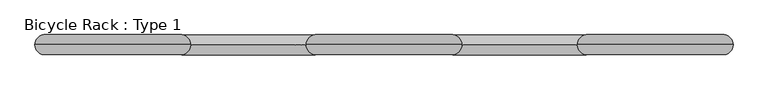
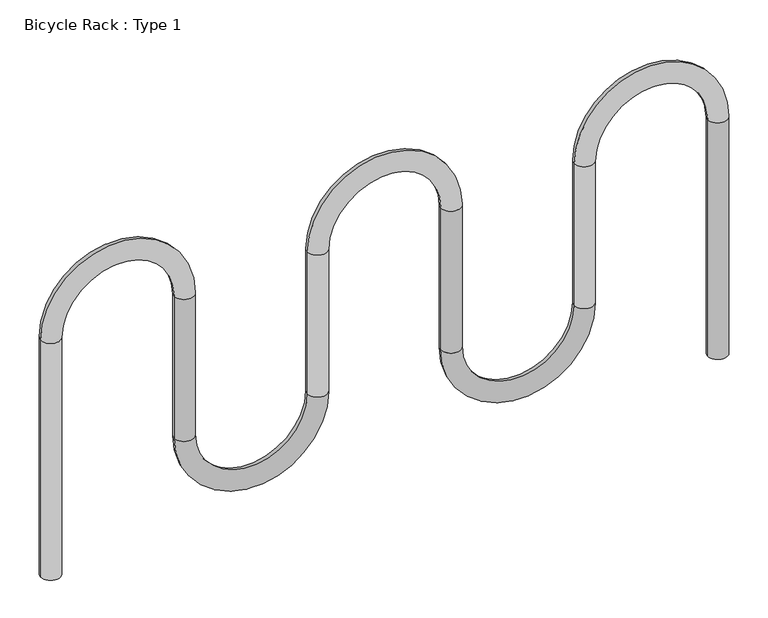
"""IFC4 building model written with IfcOpenShell, lengths in millimetres: proxy geometry, Bicycle Rack : Type 1."""

from ifc_helpers import new_model, si_unit, point, frame, origin, place, context, project, spatial, circle_curve, ellipse_curve, trimmed, source, transform, mapped, element, save
from ifc_brep_helpers import plane_surface, cylinder_surface, revolved_surface, advanced_brep


def bicycle_rack_type_1_69598307(model_context):
    return source(origin(), model_context, "Body", "AdvancedBrep", [
        advanced_brep(
        [(-985.8375, 0.0, 0.0), (-1046.1625, 0.0, 0.0), (-985.8375, 0.0, 762.0), (-1046.1625, 0.0, 762.0), (-579.4375, 0.0, 762.0), (-639.7625, 0.0, 762.0), (-639.7625, 0.0, 304.8), (-579.4375, 0.0, 304.8), (-233.3625, 0.0, 304.8), (-173.0375, 0.0, 304.8), (-173.0375, 0.0, 762.0), (-233.3625, 0.0, 762.0), (233.3625, 0.0, 762.0), (173.0375, 0.0, 762.0), (173.0375, 0.0, 304.8), (233.3625, 0.0, 304.8), (579.4375, 0.0, 304.8), (639.7625, 0.0, 304.8), (639.7625, 0.0, 762.0), (579.4375, 0.0, 762.0), (1046.1625, 0.0, 762.0), (985.8375, 0.0, 762.0), (985.8375, 0.0, 0.0), (1046.1625, 0.0, 0.0)],
        [
            (0, 1, circle_curve(frame((-1016.0, 0.0, 0.0), z_axis=(0.0, 0.0, -1.0), x_axis=(-1.0, 0.0, 0.0)), 30.1625)),
            (1, 0, circle_curve(frame((-1016.0, 0.0, 0.0), z_axis=(0.0, 0.0, -1.0), x_axis=(-1.0, 0.0, 0.0)), 30.1625)),
            (0, 2),
            (2, 3, circle_curve(frame((-1016.0, 0.0, 762.0), z_axis=(0.0, 0.0, -1.0), x_axis=(-1.0, 0.0, 0.0)), 30.1625)),
            (3, 1),
            (3, 2, circle_curve(frame((-1016.0, 0.0, 762.0), z_axis=(0.0, 0.0, -1.0), x_axis=(-1.0, 0.0, 0.0)), 30.1625)),
            (4, 3, circle_curve(frame((-812.8, 0.0, 762.0), z_axis=(0.0, -1.0, 0.0), x_axis=(-1.0, 0.0, 0.0)), 233.3625)),
            (2, 5, circle_curve(frame((-812.8, 0.0, 762.0), z_axis=(0.0, 1.0, 0.0), x_axis=(-1.0, 0.0, 0.0)), 173.0375)),
            (5, 4, circle_curve(frame((-609.6, 0.0, 762.0), z_axis=(0.0, 0.0, 1.0), x_axis=(1.0, 0.0, 0.0)), 30.1625)),
            (4, 5, circle_curve(frame((-609.6, 0.0, 762.0), z_axis=(0.0, 0.0, 1.0), x_axis=(1.0, 0.0, 0.0)), 30.1625)),
            (5, 6),
            (6, 7, circle_curve(frame((-609.6, 0.0, 304.8), z_axis=(0.0, 0.0, 1.0), x_axis=(1.0, 0.0, 0.0)), 30.1625)),
            (7, 4),
            (7, 6, circle_curve(frame((-609.6, 0.0, 304.8), z_axis=(0.0, 0.0, 1.0), x_axis=(1.0, 0.0, 0.0)), 30.1625)),
            (8, 7, circle_curve(frame((-406.4, 0.0, 304.8), z_axis=(0.0, 1.0, 0.0), x_axis=(-1.0, 0.0, 0.0)), 173.0375)),
            (6, 9, circle_curve(frame((-406.4, 0.0, 304.8), z_axis=(0.0, -1.0, 0.0), x_axis=(-1.0, 0.0, 0.0)), 233.3625)),
            (9, 8, circle_curve(frame((-203.2, 0.0, 304.8), z_axis=(0.0, 0.0, -1.0), x_axis=(-1.0, 0.0, 0.0)), 30.1625)),
            (8, 9, circle_curve(frame((-203.2, 0.0, 304.8), z_axis=(0.0, 0.0, -1.0), x_axis=(-1.0, 0.0, 0.0)), 30.1625)),
            (9, 10),
            (10, 11, circle_curve(frame((-203.2, 0.0, 762.0), z_axis=(0.0, 0.0, -1.0), x_axis=(-1.0, 0.0, 0.0)), 30.1625)),
            (11, 8),
            (11, 10, circle_curve(frame((-203.2, 0.0, 762.0), z_axis=(0.0, 0.0, -1.0), x_axis=(-1.0, 0.0, 0.0)), 30.1625)),
            (12, 11, circle_curve(frame((0.0, 0.0, 762.0), z_axis=(0.0, -1.0, 0.0), x_axis=(-1.0, 0.0, 0.0)), 233.3625)),
            (10, 13, circle_curve(frame((0.0, 0.0, 762.0), z_axis=(0.0, 1.0, 0.0), x_axis=(-1.0, 0.0, 0.0)), 173.0375)),
            (13, 12, circle_curve(frame((203.2, 0.0, 762.0), z_axis=(0.0, 0.0, 1.0), x_axis=(1.0, 0.0, 0.0)), 30.1625)),
            (12, 13, circle_curve(frame((203.2, 0.0, 762.0), z_axis=(0.0, 0.0, 1.0), x_axis=(1.0, 0.0, 0.0)), 30.1625)),
            (13, 14),
            (14, 15, circle_curve(frame((203.2, 0.0, 304.8), z_axis=(0.0, 0.0, 1.0), x_axis=(1.0, 0.0, 0.0)), 30.1625)),
            (15, 12),
            (15, 14, circle_curve(frame((203.2, 0.0, 304.8), z_axis=(0.0, 0.0, 1.0), x_axis=(1.0, 0.0, 0.0)), 30.1625)),
            (16, 15, circle_curve(frame((406.4, 0.0, 304.8), z_axis=(0.0, 1.0, 0.0), x_axis=(-1.0, 0.0, 0.0)), 173.0375)),
            (14, 17, circle_curve(frame((406.4, 0.0, 304.8), z_axis=(0.0, -1.0, 0.0), x_axis=(-1.0, 0.0, 0.0)), 233.3625)),
            (17, 16, circle_curve(frame((609.6, 0.0, 304.8), z_axis=(0.0, 0.0, -1.0), x_axis=(-1.0, 0.0, 0.0)), 30.1625)),
            (16, 17, circle_curve(frame((609.6, 0.0, 304.8), z_axis=(0.0, 0.0, -1.0), x_axis=(-1.0, 0.0, 0.0)), 30.1625)),
            (17, 18),
            (18, 19, circle_curve(frame((609.6, 0.0, 762.0), z_axis=(0.0, 0.0, -1.0), x_axis=(-1.0, 0.0, 0.0)), 30.1625)),
            (19, 16),
            (19, 18, circle_curve(frame((609.6, 0.0, 762.0), z_axis=(0.0, 0.0, -1.0), x_axis=(-1.0, 0.0, 0.0)), 30.1625)),
            (20, 19, circle_curve(frame((812.8, 0.0, 762.0), z_axis=(0.0, -1.0, 0.0), x_axis=(-1.0, 0.0, 0.0)), 233.3625)),
            (18, 21, circle_curve(frame((812.8, 0.0, 762.0), z_axis=(0.0, 1.0, 0.0), x_axis=(-1.0, 0.0, 0.0)), 173.0375)),
            (21, 20, circle_curve(frame((1016.0, 0.0, 762.0), z_axis=(0.0, 0.0, 1.0), x_axis=(1.0, 0.0, 0.0)), 30.1625)),
            (20, 21, circle_curve(frame((1016.0, 0.0, 762.0), z_axis=(0.0, 0.0, 1.0), x_axis=(1.0, 0.0, 0.0)), 30.1625)),
            (22, 23, circle_curve(frame((1016.0, 0.0, 0.0), z_axis=(0.0, 0.0, -1.0), x_axis=(1.0, 0.0, 0.0)), 30.1625)),
            (23, 22, circle_curve(frame((1016.0, 0.0, 0.0), z_axis=(0.0, 0.0, -1.0), x_axis=(1.0, 0.0, 0.0)), 30.1625)),
            (21, 22),
            (23, 20),
        ],
        [
            plane_surface(frame((-1016.0, 0.0, 0.0), z_axis=(0.0, 0.0, -1.0), x_axis=(0.0, -1.0, 0.0))),
            cylinder_surface(frame((-1016.0, 0.0, 0.0), z_axis=(0.0, 0.0, -1.0), x_axis=(-1.0, 0.0, 0.0)), 30.1625),
            revolved_surface(trimmed(ellipse_curve(frame((-1016.0, 0.0, 762.0), z_axis=(0.0, 0.0, -1.0), x_axis=(-1.0, 0.0, 0.0)), 30.1625, 30.1625), [point((-985.8375, 0.0, 762.0))], [point((-1046.1625, 0.0, 762.0))], True, "CARTESIAN"), (-812.8, 0.0, 762.0), (0.0, 1.0, 0.0)),
            revolved_surface(trimmed(ellipse_curve(frame((-1016.0, 0.0, 762.0), z_axis=(0.0, 0.0, -1.0), x_axis=(-1.0, 0.0, 0.0)), 30.1625, 30.1625), [point((-1046.1625, 0.0, 762.0))], [point((-985.8375, 0.0, 762.0))], True, "CARTESIAN"), (-812.8, 0.0, 762.0), (0.0, 1.0, 0.0)),
            cylinder_surface(frame((-609.6, 0.0, 762.0), z_axis=(0.0, 0.0, 1.0), x_axis=(1.0, 0.0, 0.0)), 30.1625),
            revolved_surface(trimmed(ellipse_curve(frame((-609.6, 0.0, 304.8), z_axis=(0.0, 0.0, 1.0), x_axis=(1.0, 0.0, 0.0)), 30.1625, 30.1625), [point((-639.7625, 0.0, 304.8))], [point((-579.4375, 0.0, 304.8))], True, "CARTESIAN"), (-406.4, 0.0, 304.8), (0.0, -1.0, 0.0)),
            revolved_surface(trimmed(ellipse_curve(frame((-609.6, 0.0, 304.8), z_axis=(0.0, 0.0, 1.0), x_axis=(1.0, 0.0, 0.0)), 30.1625, 30.1625), [point((-579.4375, 0.0, 304.8))], [point((-639.7625, 0.0, 304.8))], True, "CARTESIAN"), (-406.4, 0.0, 304.8), (0.0, -1.0, 0.0)),
            cylinder_surface(frame((-203.2, 0.0, 304.8), z_axis=(0.0, 0.0, -1.0), x_axis=(-1.0, 0.0, 0.0)), 30.1625),
            revolved_surface(trimmed(ellipse_curve(frame((-203.2, 0.0, 762.0), z_axis=(0.0, 0.0, -1.0), x_axis=(-1.0, 0.0, 0.0)), 30.1625, 30.1625), [point((-173.0375, 0.0, 762.0))], [point((-233.3625, 0.0, 762.0))], True, "CARTESIAN"), (0.0, 0.0, 762.0), (0.0, 1.0, 0.0)),
            revolved_surface(trimmed(ellipse_curve(frame((-203.2, 0.0, 762.0), z_axis=(0.0, 0.0, -1.0), x_axis=(-1.0, 0.0, 0.0)), 30.1625, 30.1625), [point((-233.3625, 0.0, 762.0))], [point((-173.0375, 0.0, 762.0))], True, "CARTESIAN"), (0.0, 0.0, 762.0), (0.0, 1.0, 0.0)),
            cylinder_surface(frame((203.2, 0.0, 762.0), z_axis=(0.0, 0.0, 1.0), x_axis=(1.0, 0.0, 0.0)), 30.1625),
            revolved_surface(trimmed(ellipse_curve(frame((203.2, 0.0, 304.8), z_axis=(0.0, 0.0, 1.0), x_axis=(1.0, 0.0, 0.0)), 30.1625, 30.1625), [point((173.0375, 0.0, 304.8))], [point((233.3625, 0.0, 304.8))], True, "CARTESIAN"), (406.4, 0.0, 304.8), (0.0, -1.0, 0.0)),
            revolved_surface(trimmed(ellipse_curve(frame((203.2, 0.0, 304.8), z_axis=(0.0, 0.0, 1.0), x_axis=(1.0, 0.0, 0.0)), 30.1625, 30.1625), [point((233.3625, 0.0, 304.8))], [point((173.0375, 0.0, 304.8))], True, "CARTESIAN"), (406.4, 0.0, 304.8), (0.0, -1.0, 0.0)),
            cylinder_surface(frame((609.6, 0.0, 304.8), z_axis=(0.0, 0.0, -1.0), x_axis=(-1.0, 0.0, 0.0)), 30.1625),
            revolved_surface(trimmed(ellipse_curve(frame((609.6, 0.0, 762.0), z_axis=(0.0, 0.0, -1.0), x_axis=(-1.0, 0.0, 0.0)), 30.1625, 30.1625), [point((639.7625, 0.0, 762.0))], [point((579.4375, 0.0, 762.0))], True, "CARTESIAN"), (812.8, 0.0, 762.0), (0.0, 1.0, 0.0)),
            revolved_surface(trimmed(ellipse_curve(frame((609.6, 0.0, 762.0), z_axis=(0.0, 0.0, -1.0), x_axis=(-1.0, 0.0, 0.0)), 30.1625, 30.1625), [point((579.4375, 0.0, 762.0))], [point((639.7625, 0.0, 762.0))], True, "CARTESIAN"), (812.8, 0.0, 762.0), (0.0, 1.0, 0.0)),
            plane_surface(frame((1016.0, 0.0, 0.0), z_axis=(0.0, 0.0, -1.0), x_axis=(0.0, -1.0, 0.0))),
            cylinder_surface(frame((1016.0, 0.0, 762.0), z_axis=(0.0, 0.0, 1.0), x_axis=(1.0, 0.0, 0.0)), 30.1625),
        ],
        [
            (0, [[1, 2]]),
            (1, [[-1, 3, 4, 5]]),
            (1, [[-2, -5, 6, -3]]),
            (2, [[7, -4, 8, 9]]),
            (3, [[-8, -6, -7, 10]]),
            (4, [[-9, 11, 12, 13]]),
            (4, [[-10, -13, 14, -11]]),
            (5, [[15, -12, 16, 17]]),
            (6, [[-16, -14, -15, 18]]),
            (7, [[-17, 19, 20, 21]]),
            (7, [[-18, -21, 22, -19]]),
            (8, [[23, -20, 24, 25]]),
            (9, [[-24, -22, -23, 26]]),
            (10, [[-25, 27, 28, 29]]),
            (10, [[-26, -29, 30, -27]]),
            (11, [[31, -28, 32, 33]]),
            (12, [[-32, -30, -31, 34]]),
            (13, [[-33, 35, 36, 37]]),
            (13, [[-34, -37, 38, -35]]),
            (14, [[39, -36, 40, 41]]),
            (15, [[-40, -38, -39, 42]]),
            (16, [[43, 44]]),
            (17, [[-41, 45, -44, 46]]),
            (17, [[-42, -46, -43, -45]]),
        ],
    ),
    ])


if __name__ == "__main__":
    model = new_model("IFC4")
    model_context = context("Model", 3, world=origin())
    ifc_project = project(units=[si_unit("LENGTHUNIT", "METRE", prefix="MILLI")], contexts=[model_context])
    site = spatial("IfcSite", under=ifc_project)
    building = spatial("IfcBuilding", under=site)
    placement = place(None, origin())
    bicycle_rack_type_1_shape = bicycle_rack_type_1_69598307(model_context)
    element("IfcBuildingElementProxy", 1, Name="Bicycle Rack : Type 1", ObjectType="Bicycle Rack : Type 1", at=placement, inside=building, context=model_context, shape_type="MappedRepresentation", body=[
        mapped(bicycle_rack_type_1_shape, transform((0.0, 0.0, 0.0), x_axis=(1.0, 0.0, 0.0), y_axis=(0.0, 1.0, 0.0), z_axis=(0.0, 0.0, 1.0))),
    ])
    save(model, "model.ifc")

# Revit data of these elements
# Type "Bicycle Rack : Type 1"
#   Default Elevation = 0
